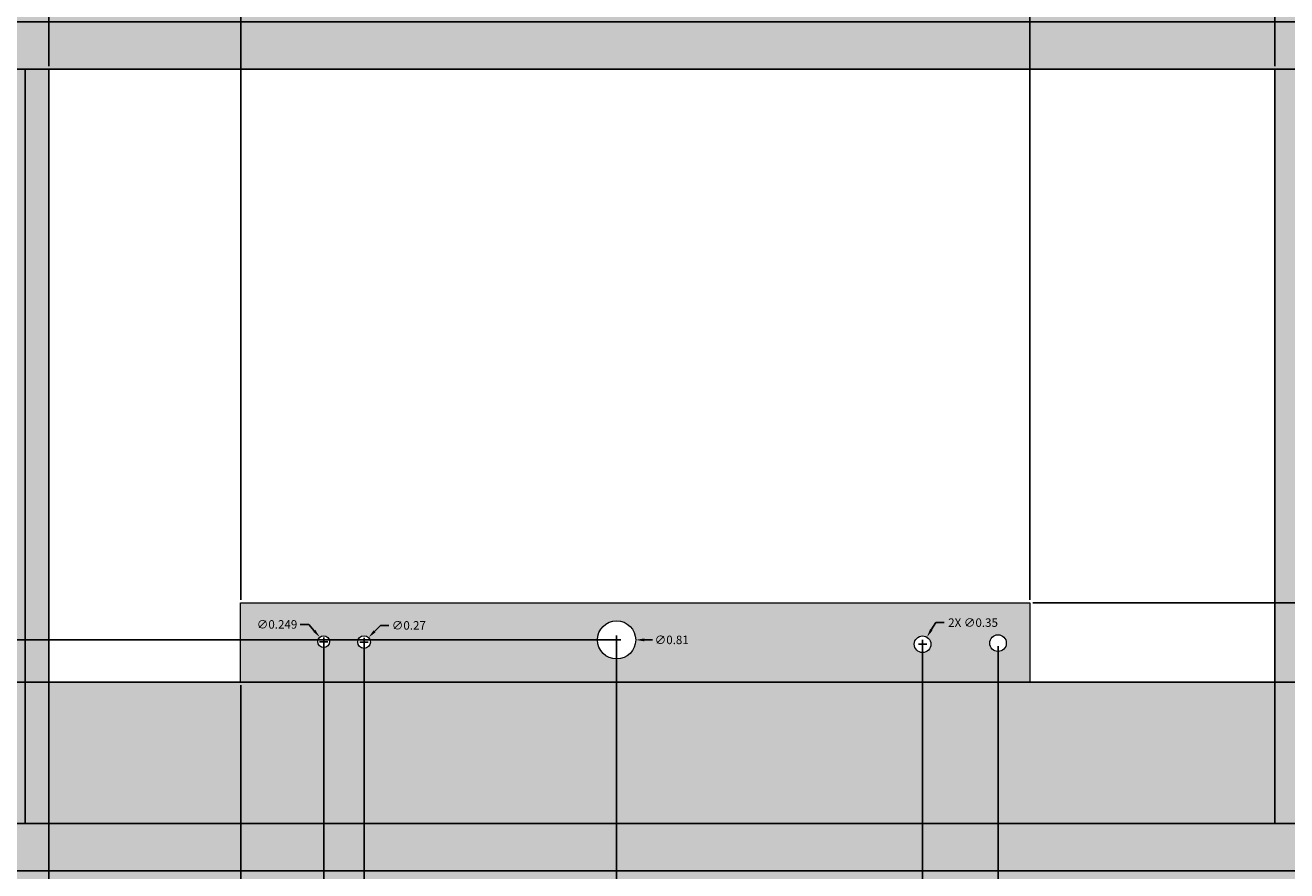
# Model space of a CAD drawing. Units: inches. Extents: x 4508 to 4723, y 847 to 1020.
# Tile 7 of 32: x 4604 to 4631, y 887 to 905. Entities that reach past the tile are written whole.
import ezdxf

# ---------------------------------------------------------------- set-up
doc = ezdxf.new("R2010")
doc.units = ezdxf.units.IN
for name, color, linetype, lineweight in [('A-ANNO-DIMS', 2, 'Continuous', 18), ('A-ANNO-NPLT', 8, 'Continuous', 13), ('A-EQPM', 4, 'Continuous', 18), ('A-FURN', 8, 'Continuous', 25), ('A-WALL-PATT', 254, 'Continuous', 13)]:
    doc.layers.add(name, color=color, linetype=linetype, lineweight=lineweight)
doc.styles.get("Standard").update_dxf_attribs({"font": 'arial.ttf'})
doc.dimstyles.get("Standard").update_dxf_attribs({"dimtxt": 0.18, "dimasz": 0.18, "dimexe": 0.18, "dimexo": 0.0625, "dimgap": 0.09, "dimtad": 0, "dimtih": 1, "dimtoh": 1, "dimdec": 4, "dimzin": 0, "dimdsep": 46, "dimtxsty": 'Standard', "dimcen": 0.09, "dimadec": 0, "dimazin": 0, "dimtfac": 1, "dimtdec": 4, "dimtofl": 0, "dimtmove": 0, "dimatfit": 3, "dimfxl": 1, "dimtolj": 1, "dimtzin": 0, "dimarcsym": 0})

# ---------------------------------------------------------------- blocks, each defined once
blk = doc.blocks.new('*D30')
at = {"layer": 'A-ANNO-DIMS', "color": 0, "lineweight": -2, "transparency": 16777216}
for p, q in [((4604.494, 903.809), (4604.494, 1002.877)), ((4630.494, 903.809), (4630.494, 1002.877)), ((4604.674, 1002.697), (4617.273, 1002.697)), ((4630.314, 1002.697), (4617.714, 1002.697))]:
    blk.add_line(p, q, dxfattribs=at)
at = {"layer": 'A-ANNO-DIMS', "color": 0, "lineweight": 9, "transparency": 16777216}
for points in [[(4604.674, 1002.727), (4604.674, 1002.667), (4604.494, 1002.697)], [(4630.314, 1002.727), (4630.314, 1002.667), (4630.494, 1002.697)]]:
    blk.add_solid(points, dxfattribs=at)
at = {"layer": 'Defpoints', "color": 0, "lineweight": 9, "transparency": 16777216}
for p in [(4630.494, 1002.697), (4604.494, 903.747), (4630.494, 903.747)]:
    blk.add_point(p, dxfattribs=at)
at = {"layer": 'A-ANNO-DIMS', "color": 0, "transparency": 16777216, "insert": (4617.494, 1002.697), "char_height": 0.18, "attachment_point": 5}
blk.add_mtext('\\A1;26', dxfattribs=at)
blk = doc.blocks.new('*D32')
at = {"layer": 'A-ANNO-DIMS', "color": 0, "lineweight": -2, "transparency": 16777216}
for p, q in [((4604.431, 890.747), (4532.864, 890.747)), ((4533.044, 890.567), (4533.044, 889.429)), ((4533.044, 887.927), (4533.044, 889.065)), ((4604.431, 887.747), (4532.864, 887.747))]:
    blk.add_line(p, q, dxfattribs=at)
at = {"layer": 'A-ANNO-DIMS', "color": 0, "lineweight": 9, "transparency": 16777216}
for points in [[(4533.014, 890.567), (4533.074, 890.567), (4533.044, 890.747)], [(4533.014, 887.927), (4533.074, 887.927), (4533.044, 887.747)]]:
    blk.add_solid(points, dxfattribs=at)
at = {"layer": 'Defpoints', "color": 0, "lineweight": 9, "transparency": 16777216}
for p in [(4533.044, 890.747), (4604.494, 890.747), (4604.494, 887.747)]:
    blk.add_point(p, dxfattribs=at)
at = {"layer": 'A-ANNO-DIMS', "color": 0, "transparency": 16777216, "insert": (4533.044, 889.247), "char_height": 0.18, "attachment_point": 5}
blk.add_mtext('\\A1;3', dxfattribs=at)
blk = doc.blocks.new('*D33')
at = {"layer": 'A-ANNO-DIMS', "color": 0, "lineweight": -2, "transparency": 16777216}
for p, q in [((4604.494, 890.684), (4604.494, 866.617)), ((4608.562, 890.684), (4608.562, 866.617)), ((4604.674, 866.797), (4606.13, 866.797)), ((4608.382, 866.797), (4606.925, 866.797))]:
    blk.add_line(p, q, dxfattribs=at)
at = {"layer": 'A-ANNO-DIMS', "color": 0, "lineweight": 9, "transparency": 16777216}
for points in [[(4604.674, 866.827), (4604.674, 866.767), (4604.494, 866.797)], [(4608.382, 866.827), (4608.382, 866.767), (4608.562, 866.797)]]:
    blk.add_solid(points, dxfattribs=at)
at = {"layer": 'Defpoints', "color": 0, "lineweight": 9, "transparency": 16777216}
for p in [(4604.494, 890.747), (4608.562, 890.747), (4608.562, 866.797)]:
    blk.add_point(p, dxfattribs=at)
at = {"layer": 'A-ANNO-DIMS', "color": 0, "transparency": 16777216, "insert": (4606.528, 866.797), "char_height": 0.18, "attachment_point": 5}
blk.add_mtext('\\A1;4.068', dxfattribs=at)
blk = doc.blocks.new('*D34')
at = {"layer": 'A-ANNO-DIMS', "color": 0, "lineweight": -2, "transparency": 16777216}
for p, q in [((4608.562, 892.49), (4608.562, 1002.877)), ((4625.298, 892.49), (4625.298, 1002.877)), ((4608.742, 1002.697), (4616.475, 1002.697)), ((4625.118, 1002.697), (4617.385, 1002.697))]:
    blk.add_line(p, q, dxfattribs=at)
at = {"layer": 'A-ANNO-DIMS', "color": 0, "lineweight": 9, "transparency": 16777216}
for points in [[(4608.742, 1002.727), (4608.742, 1002.667), (4608.562, 1002.697)], [(4625.118, 1002.727), (4625.118, 1002.667), (4625.298, 1002.697)]]:
    blk.add_solid(points, dxfattribs=at)
at = {"layer": 'Defpoints', "color": 0, "lineweight": 9, "transparency": 16777216}
for p in [(4625.298, 1002.697), (4608.562, 892.428), (4625.298, 892.428)]:
    blk.add_point(p, dxfattribs=at)
at = {"layer": 'A-ANNO-DIMS', "color": 0, "transparency": 16777216, "insert": (4616.93, 1002.697), "char_height": 0.18, "attachment_point": 5}
blk.add_mtext('\\A1;16.737', dxfattribs=at)
blk = doc.blocks.new('*D35')
at = {"layer": 'A-ANNO-DIMS', "color": 0, "lineweight": -2, "transparency": 16777216}
for p, q in [((4625.361, 892.428), (4702.124, 892.428)), ((4701.944, 892.248), (4701.944, 891.769)), ((4701.944, 890.927), (4701.944, 891.405)), ((4625.361, 890.747), (4702.124, 890.747))]:
    blk.add_line(p, q, dxfattribs=at)
at = {"layer": 'A-ANNO-DIMS', "color": 0, "lineweight": 9, "transparency": 16777216}
for points in [[(4701.914, 892.248), (4701.974, 892.248), (4701.944, 892.428)], [(4701.914, 890.927), (4701.974, 890.927), (4701.944, 890.747)]]:
    blk.add_solid(points, dxfattribs=at)
at = {"layer": 'Defpoints', "color": 0, "lineweight": 9, "transparency": 16777216}
for p in [(4625.298, 892.428), (4701.944, 892.428), (4625.298, 890.747)]:
    blk.add_point(p, dxfattribs=at)
at = {"layer": 'A-ANNO-DIMS', "color": 0, "transparency": 16777216, "insert": (4701.944, 891.587), "char_height": 0.18, "attachment_point": 5}
blk.add_mtext('\\A1;1.681', dxfattribs=at)
blk = doc.blocks.new('*D36')
at = {"layer": 'A-ANNO-DIMS', "color": 0, "lineweight": -2, "transparency": 16777216}
for p, q in [((4610.322, 891.543), (4610.322, 866.617)), ((4608.562, 890.684), (4608.562, 866.617)), ((4608.742, 866.797), (4609.127, 866.797)), ((4610.142, 866.797), (4609.757, 866.797))]:
    blk.add_line(p, q, dxfattribs=at)
at = {"layer": 'A-ANNO-DIMS', "color": 0, "lineweight": 9, "transparency": 16777216}
for points in [[(4608.742, 866.827), (4608.742, 866.767), (4608.562, 866.797)], [(4610.142, 866.827), (4610.142, 866.767), (4610.322, 866.797)]]:
    blk.add_solid(points, dxfattribs=at)
at = {"layer": 'Defpoints', "color": 0, "lineweight": 9, "transparency": 16777216}
for p in [(4610.322, 891.605), (4608.562, 890.747), (4610.322, 866.797)]:
    blk.add_point(p, dxfattribs=at)
at = {"layer": 'A-ANNO-DIMS', "color": 0, "transparency": 16777216, "insert": (4609.442, 866.797), "char_height": 0.18, "attachment_point": 5}
blk.add_mtext('\\A1;1.76', dxfattribs=at)
blk = doc.blocks.new('*D37')
at = {"layer": 'A-ANNO-DIMS', "color": 0, "lineweight": -2, "transparency": 16777216}
for p, q in [((4610.322248, 891.542903), (4610.322248, 866.616874)), ((4611.179162, 891.534506), (4611.179162, 866.616874)), ((4610.142248, 866.796874), (4609.962248, 866.796874)), ((4611.359162, 866.796874), (4611.539162, 866.796874))]:
    blk.add_line(p, q, dxfattribs=at)
at = {"layer": 'A-ANNO-DIMS', "color": 0, "lineweight": 9, "transparency": 16777216}
for points in [[(4610.142248, 866.826874), (4610.142248, 866.766874), (4610.322248, 866.796874)], [(4611.359162, 866.826874), (4611.359162, 866.766874), (4611.179162, 866.796874)]]:
    blk.add_solid(points, dxfattribs=at)
at = {"layer": 'Defpoints', "color": 0, "lineweight": 9, "transparency": 16777216}
for p in [(4610.322248, 891.605403), (4611.179162, 891.597006), (4611.179162, 866.796874)]:
    blk.add_point(p, dxfattribs=at)
at = {"layer": 'A-ANNO-DIMS', "color": 0, "transparency": 16777216, "insert": (4610.750705, 866.796874), "char_height": 0.18, "attachment_point": 5}
blk.add_mtext('\\A1;0.857', dxfattribs=at)
blk = doc.blocks.new('*D38')
at = {"layer": 'A-ANNO-DIMS', "color": 0, "lineweight": -2, "transparency": 16777216}
for p, q in [((4616.533, 891.581), (4616.533, 866.617)), ((4611.179, 891.535), (4611.179, 866.617)), ((4611.359, 866.797), (4613.463, 866.797)), ((4616.353, 866.797), (4614.249, 866.797))]:
    blk.add_line(p, q, dxfattribs=at)
at = {"layer": 'A-ANNO-DIMS', "color": 0, "lineweight": 9, "transparency": 16777216}
for points in [[(4611.359, 866.827), (4611.359, 866.767), (4611.179, 866.797)], [(4616.353, 866.827), (4616.353, 866.767), (4616.533, 866.797)]]:
    blk.add_solid(points, dxfattribs=at)
at = {"layer": 'Defpoints', "color": 0, "lineweight": 9, "transparency": 16777216}
for p in [(4611.179, 891.597), (4616.533, 891.643), (4616.533, 866.797)]:
    blk.add_point(p, dxfattribs=at)
at = {"layer": 'A-ANNO-DIMS', "color": 0, "transparency": 16777216, "insert": (4613.856, 866.797), "char_height": 0.18, "attachment_point": 5}
blk.add_mtext('\\A1;5.354', dxfattribs=at)
blk = doc.blocks.new('*D39')
at = {"layer": 'A-ANNO-DIMS', "color": 0, "lineweight": -2, "transparency": 16777216}
for p, q in [((4616.533, 891.581), (4616.533, 866.617)), ((4623.022, 891.488), (4623.022, 866.617)), ((4616.713, 866.797), (4619.383, 866.797)), ((4622.842, 866.797), (4620.172, 866.797))]:
    blk.add_line(p, q, dxfattribs=at)
at = {"layer": 'A-ANNO-DIMS', "color": 0, "lineweight": 9, "transparency": 16777216}
for points in [[(4616.713, 866.827), (4616.713, 866.767), (4616.533, 866.797)], [(4622.842, 866.827), (4622.842, 866.767), (4623.022, 866.797)]]:
    blk.add_solid(points, dxfattribs=at)
at = {"layer": 'Defpoints', "color": 0, "lineweight": 9, "transparency": 16777216}
for p in [(4616.533, 891.643), (4623.022, 891.551), (4623.022, 866.797)]:
    blk.add_point(p, dxfattribs=at)
at = {"layer": 'A-ANNO-DIMS', "color": 0, "transparency": 16777216, "insert": (4619.777, 866.797), "char_height": 0.18, "attachment_point": 5}
blk.add_mtext('\\A1;6.489', dxfattribs=at)
blk = doc.blocks.new('*D40')
at = {"layer": 'A-ANNO-DIMS', "color": 0, "lineweight": -2, "transparency": 16777216}
for p, q in [((4623.022, 891.488), (4623.022, 866.617)), ((4624.621, 891.511), (4624.621, 866.617)), ((4623.202, 866.797), (4623.436, 866.797)), ((4624.441, 866.797), (4624.207, 866.797))]:
    blk.add_line(p, q, dxfattribs=at)
at = {"layer": 'A-ANNO-DIMS', "color": 0, "lineweight": 9, "transparency": 16777216}
for points in [[(4623.202, 866.827), (4623.202, 866.767), (4623.022, 866.797)], [(4624.441, 866.827), (4624.441, 866.767), (4624.621, 866.797)]]:
    blk.add_solid(points, dxfattribs=at)
at = {"layer": 'Defpoints', "color": 0, "lineweight": 9, "transparency": 16777216}
for p in [(4623.022, 891.551), (4624.621, 891.574), (4624.621, 866.797)]:
    blk.add_point(p, dxfattribs=at)
at = {"layer": 'A-ANNO-DIMS', "color": 0, "transparency": 16777216, "insert": (4623.821, 866.797), "char_height": 0.18, "attachment_point": 5}
blk.add_mtext('\\A1;1.599', dxfattribs=at)
blk = doc.blocks.new('*D41')
at = {"layer": 'A-ANNO-DIMS', "color": 0, "lineweight": -2, "transparency": 16777216}
for p, q in [((4616.47, 891.643), (4532.864, 891.643)), ((4533.044, 891.643), (4533.044, 891.823)), ((4533.044, 891.823), (4533.224, 891.823)), ((4533.044, 890.927), (4533.044, 891.463)), ((4608.499, 890.747), (4532.864, 890.747))]:
    blk.add_line(p, q, dxfattribs=at)
at = {"layer": 'A-ANNO-DIMS', "color": 0, "lineweight": 9, "transparency": 16777216}
for points in [[(4533.014, 891.463), (4533.074, 891.463), (4533.044, 891.643)], [(4533.014, 890.927), (4533.074, 890.927), (4533.044, 890.747)]]:
    blk.add_solid(points, dxfattribs=at)
at = {"layer": 'Defpoints', "color": 0, "lineweight": 9, "transparency": 16777216}
for p in [(4533.044, 891.643), (4616.533, 891.643), (4608.562, 890.747)]:
    blk.add_point(p, dxfattribs=at)
at = {"layer": 'A-ANNO-DIMS', "color": 0, "transparency": 16777216, "insert": (4533.547, 891.823), "char_height": 0.18, "attachment_point": 5}
blk.add_mtext('\\A1;0.90', dxfattribs=at)
blk = doc.blocks.new('*D48')
at = {"layer": 'A-ANNO-DIMS', "color": 0, "lineweight": -2, "transparency": 16777216}
for p, q in [((4616.443, 891.643), (4616.623, 891.643)), ((4616.533, 891.553), (4616.533, 891.733)), ((4617.298, 891.643), (4617.118, 891.643))]:
    blk.add_line(p, q, dxfattribs=at)
at = {"layer": 'A-ANNO-DIMS', "color": 0, "lineweight": 9, "transparency": 16777216}
blk.add_solid([(4617.118, 891.673), (4617.118, 891.613), (4616.938, 891.643)], dxfattribs=at)
at = {"layer": 'Defpoints', "color": 0, "lineweight": 9, "transparency": 16777216}
for p in [(4616.128, 891.644), (4616.938, 891.643)]:
    blk.add_point(p, dxfattribs=at)
at = {"layer": 'A-ANNO-DIMS', "color": 0, "transparency": 16777216, "insert": (4617.702, 891.643), "char_height": 0.18, "attachment_point": 5}
blk.add_mtext('\\A1;∅0.81', dxfattribs=at)
blk = doc.blocks.new('*D49')
at = {"layer": 'A-ANNO-DIMS', "color": 0, "lineweight": -2, "transparency": 16777216}
for p, q in [((4609.824, 891.971), (4610.004, 891.971)), ((4610.004, 891.971), (4610.122, 891.835)), ((4610.232, 891.605), (4610.412, 891.605)), ((4610.322, 891.515), (4610.322, 891.695))]:
    blk.add_line(p, q, dxfattribs=at)
at = {"layer": 'A-ANNO-DIMS', "color": 0, "lineweight": 9, "transparency": 16777216}
blk.add_solid([(4610.145, 891.855), (4610.1, 891.816), (4610.241, 891.699)], dxfattribs=at)
at = {"layer": 'Defpoints', "color": 0, "lineweight": 9, "transparency": 16777216}
for p in [(4610.241, 891.699), (4610.404, 891.511)]:
    blk.add_point(p, dxfattribs=at)
at = {"layer": 'A-ANNO-DIMS', "color": 0, "transparency": 16777216, "insert": (4609.333, 891.971), "char_height": 0.18, "attachment_point": 5}
blk.add_mtext('\\A1;∅0.249', dxfattribs=at)
blk = doc.blocks.new('*D50')
at = {"layer": 'A-ANNO-DIMS', "color": 0, "lineweight": -2, "transparency": 16777216}
for p, q in [((4611.526, 891.95), (4611.4, 891.822)), ((4611.706, 891.95), (4611.526, 891.95)), ((4611.089, 891.597), (4611.269, 891.597)), ((4611.179, 891.507), (4611.179, 891.687))]:
    blk.add_line(p, q, dxfattribs=at)
at = {"layer": 'A-ANNO-DIMS', "color": 0, "lineweight": 9, "transparency": 16777216}
blk.add_solid([(4611.378, 891.843), (4611.421, 891.801), (4611.274, 891.693)], dxfattribs=at)
at = {"layer": 'Defpoints', "color": 0, "lineweight": 9, "transparency": 16777216}
for p in [(4611.274, 891.693), (4611.085, 891.501)]:
    blk.add_point(p, dxfattribs=at)
at = {"layer": 'A-ANNO-DIMS', "color": 0, "transparency": 16777216, "insert": (4612.128, 891.95), "char_height": 0.18, "attachment_point": 5}
blk.add_mtext('\\A1;∅0.27', dxfattribs=at)
blk = doc.blocks.new('*D51')
at = {"layer": 'A-ANNO-DIMS', "color": 0, "lineweight": -2, "transparency": 16777216}
for p, q in [((4623.299, 892.009), (4623.206, 891.855)), ((4623.479, 892.009), (4623.299, 892.009)), ((4623.022, 891.461), (4623.022, 891.641)), ((4622.932, 891.551), (4623.112, 891.551))]:
    blk.add_line(p, q, dxfattribs=at)
at = {"layer": 'A-ANNO-DIMS', "color": 0, "lineweight": 9, "transparency": 16777216}
blk.add_solid([(4623.181, 891.871), (4623.232, 891.84), (4623.113, 891.701)], dxfattribs=at)
at = {"layer": 'Defpoints', "color": 0, "lineweight": 9, "transparency": 16777216}
for p in [(4623.113, 891.701), (4622.93, 891.4)]:
    blk.add_point(p, dxfattribs=at)
at = {"layer": 'A-ANNO-DIMS', "color": 0, "transparency": 16777216, "insert": (4624.092, 892.009), "char_height": 0.18, "attachment_point": 5}
blk.add_mtext('\\A1;2X ∅0.35', dxfattribs=at)

msp = doc.modelspace()

# ---------------------------------------------------------------- hatches: boundary and pattern name
at = {"layer": 'A-WALL-PATT', "transparency": 33554508}
h = msp.add_hatch(color=256, dxfattribs=at)
h.dxf.hatch_style = 1
h.paths.add_polyline_path([(4661.6706, 954.043, -0.3739004), (4658.5765, 957.6021, -1), (4665.7646, 957.6021, -0.3739004), (4662.6706, 954.043), (4662.6706, 944.4021, -0.2114781), (4670.3062, 945.0869), (4670.3062, 968.0592, -0.4632086), (4663.3246, 973.9783, -0.4632086), (4670.3062, 979.8975), (4670.3062, 994.7469), (4588.9938, 994.7469), (4588.9938, 904.7469), (4657.9938, 904.7469), (4657.9938, 886.7469), (4549.9938, 886.7469), (4549.9938, 878.7469), (4693.9938, 878.7469), (4693.9938, 994.7469), (4671.8062, 994.7469), (4671.8062, 979.4411, -0.2941682), (4675.3246, 973.9783, -0.2941682), (4671.8062, 968.5156), (4671.8062, 944.4278, -0.2741114), (4676.7298, 936.1217, -0.2741114), (4671.8062, 927.8155), (4671.8062, 907.6998, -0.3779645), (4677.0562, 901.7469, -0.3779645), (4671.8062, 895.7939), (4671.8062, 883.7469), (4670.3062, 883.7469), (4670.3062, 895.7939, -0.3779645), (4665.0562, 901.7469, -0.3779645), (4670.3062, 907.6998), (4670.3062, 927.1564, -0.2114781), (4662.6706, 927.8412), (4662.6706, 918.2003, -0.3739004), (4665.7646, 914.6412, -1), (4658.5765, 914.6412, -0.3739004), (4661.6706, 918.2003), (4661.6706, 928.4807, -0.2391825), (4657.7936, 936.1217, -0.2391825), (4661.6706, 943.7626)])
at = {"layer": 'A-WALL-PATT', "transparency": 33554681}
h = msp.add_hatch(color=256, dxfattribs=at)
h.dxf.hatch_style = 1
h.paths.add_polyline_path([(4577.4938, 903.7469), (4550.9938, 903.7469), (4550.9938, 887.7469), (4577.4938, 887.7469)], flags=0)
h.paths.add_polyline_path([(4603.9938, 903.7469), (4577.9938, 903.7469), (4577.9938, 887.7469), (4603.9938, 887.7469)], flags=0)
h.paths.add_polyline_path([(4656.9938, 903.7469), (4630.9938, 903.7469), (4630.9938, 887.7469), (4656.9938, 887.7469)], flags=0)
h.paths.add_polyline_path([(4657.9938, 904.7469), (4549.9938, 904.7469), (4549.9938, 886.7469), (4657.9938, 886.7469)])
h.paths.add_polyline_path([(4656.9938, 903.7469), (4656.9938, 887.7469), (4550.9938, 887.7469), (4550.9938, 903.7469)], flags=16)
h = msp.add_hatch(color=256, dxfattribs=at)
h.dxf.hatch_style = 1
h.paths.add_polyline_path([(4577.4938, 903.7469), (4550.9938, 903.7469), (4550.9938, 887.7469), (4577.4938, 887.7469)])
h.paths.add_polyline_path([(4603.9938, 903.7469), (4577.9938, 903.7469), (4577.9938, 887.7469), (4603.9938, 887.7469)])
h.paths.add_polyline_path([(4656.9938, 903.7469), (4630.9938, 903.7469), (4630.9938, 887.7469), (4656.9938, 887.7469)])
h = msp.add_hatch(color=256, dxfattribs=at)
h.dxf.hatch_style = 1
h.paths.add_polyline_path([(4604.4938, 903.7469), (4603.9938, 903.7469), (4603.9938, 887.7469), (4604.4938, 887.7469)])
h.paths.add_polyline_path([(4630.9938, 903.7469), (4630.4938, 903.7469), (4630.4938, 887.7469), (4630.9938, 887.7469)])
h.paths.add_polyline_path([(4577.9938, 903.7469), (4577.4938, 903.7469), (4577.4938, 887.7469), (4577.9938, 887.7469)])
at = {"layer": 'A-WALL-PATT', "transparency": 33554676}
h = msp.add_hatch(color=256, dxfattribs=at)
h.dxf.hatch_style = 1
h.paths.add_polyline_path([(4625.2983, 892.4277), (4608.5617, 892.4277), (4608.5617, 890.7469), (4625.2983, 890.7469)])
h.paths.add_polyline_path([(4616.1277, 891.6433, -1), (4616.9379, 891.6433, -1)], flags=16)
h.paths.add_polyline_path([(4611.044, 891.597, -1), (4611.3143, 891.597, -1)], flags=16)
h.paths.add_polyline_path([(4610.1977, 891.6054, -1), (4610.4468, 891.6054, -1)], flags=16)
h.paths.add_polyline_path([(4623.198, 891.5507, -1), (4622.8455, 891.5507, -1)], flags=16)
h.paths.add_polyline_path([(4624.7971, 891.5739, -1), (4624.4444, 891.5739, -1)], flags=16)
at = {"layer": 'A-WALL-PATT', "transparency": 33554681}
h = msp.add_hatch(color=256, dxfattribs=at)
h.dxf.hatch_style = 1
h.paths.add_polyline_path([(4630.4938, 890.7469), (4604.4938, 890.7469), (4604.4938, 887.7469), (4630.4938, 887.7469)])

# ---------------------------------------------------------------- linework, layer by layer
at = {"layer": 'A-ANNO-NPLT'}
for p in [(4603.9938, 895.7469), (4630.4938, 895.7469)]:
    msp.add_point(p, dxfattribs=at)
at = {"layer": 'A-EQPM'}
msp.add_lwpolyline([(4608.5617, 892.4277), (4625.2983, 892.4277), (4625.2983, 890.7469), (4608.5617, 890.7469)], close=True, dxfattribs=at)
for centre, radius in [((4616.5328, 891.6433), 0.4051), ((4610.3222, 891.6054), 0.1245), ((4611.1792, 891.597), 0.1351), ((4623.0217, 891.5507), 0.1763), ((4624.6207, 891.5739), 0.1764)]:
    msp.add_circle(centre, radius, dxfattribs=at)
at = {"layer": 'A-FURN'}
for p, q in [((4603.9938, 903.7469), (4603.9938, 887.7469)), ((4604.4938, 903.7469), (4604.4938, 887.7469)), ((4630.4938, 903.7469), (4630.4938, 887.7469)), ((4604.4938, 890.7469), (4630.4938, 890.7469))]:
    msp.add_line(p, q, dxfattribs=at)
for points in [[(4657.9938, 886.7469), (4549.9938, 886.7469), (4549.9938, 904.7469), (4657.9938, 904.7469)], [(4656.9938, 887.7469), (4550.9938, 887.7469), (4550.9938, 903.7469), (4656.9938, 903.7469)]]:
    msp.add_lwpolyline(points, close=True, dxfattribs=at)

# ---------------------------------------------------------------- dimensions: what is measured, and where the dimension line sits
at = {"layer": 'A-ANNO-DIMS'}
for base, p1, p2, override, picture, middle in [((4630.4938, 1002.6969), (4604.4938, 903.7469), (4630.4938, 903.7469), {"dimdec": 0, "dimlfac": 1, "dimrnd": 0, "dimzin": 0, "dimdsep": 46, "dimlunit": 2}, '*D30', (4617.4938, 1002.6969)), ((4625.2983, 1002.6969), (4608.5617, 892.4277), (4625.2983, 892.4277), {"dimdec": 3, "dimlfac": 1, "dimrnd": 0, "dimzin": 0, "dimdsep": 46, "dimlunit": 2}, '*D34', (4616.93, 1002.6969)), ((4610.3222, 866.7969), (4608.5617, 890.7469), (4610.3222, 891.6054), {"dimdec": 2, "dimlfac": 1, "dimrnd": 0, "dimzin": 0, "dimdsep": 46, "dimlunit": 2}, '*D36', (4609.442, 866.7969)), ((4611.1792, 866.7969), (4610.3222, 891.6054), (4611.1792, 891.597), {"dimdec": 3, "dimlfac": 1, "dimrnd": 0, "dimzin": 0, "dimdsep": 46, "dimlunit": 2}, '*D37', (4610.7507, 866.7969)), ((4616.5328, 866.7969), (4611.1792, 891.597), (4616.5328, 891.6433), {"dimdec": 3, "dimlfac": 1, "dimrnd": 0, "dimzin": 0, "dimdsep": 46, "dimlunit": 2}, '*D38', (4613.856, 866.7969)), ((4623.0217, 866.7969), (4616.5328, 891.6433), (4623.0217, 891.5507), {"dimdec": 3, "dimlfac": 1, "dimrnd": 0, "dimzin": 0, "dimdsep": 46, "dimlunit": 2}, '*D39', (4619.7773, 866.7969)), ((4624.6207, 866.7969), (4623.0217, 891.5507), (4624.6207, 891.5739), {"dimdec": 3, "dimlfac": 1, "dimrnd": 0, "dimzin": 0, "dimdsep": 46, "dimlunit": 2}, '*D40', (4623.8212, 866.7969)), ((4608.5617, 866.7969), (4604.4938, 890.7469), (4608.5617, 890.7469), {"dimdec": 3, "dimlfac": 1, "dimrnd": 0, "dimzin": 0, "dimdsep": 46, "dimlunit": 2}, '*D33', (4606.5277, 866.7969))]:
    dim = msp.add_linear_dim(base=base, p1=p1, p2=p2, dimstyle='Standard', override=override, dxfattribs=at)
    dim.commit()
    dim.dimension.update_dxf_attribs({"geometry": picture, "text_midpoint": middle})
for base, p1, p2, override, picture, middle in [((4701.9438, 892.4277), (4625.2983, 890.7469), (4625.2983, 892.4277), {"dimdec": 3, "dimlfac": 1, "dimrnd": 0, "dimzin": 0, "dimdsep": 46, "dimlunit": 2}, '*D35', (4701.9438, 891.5873)), ((4533.0438, 891.6433), (4608.5617, 890.7469), (4616.5328, 891.6433), {"dimdec": 2, "dimlfac": 1, "dimrnd": 0, "dimzin": 0, "dimdsep": 46, "dimlunit": 2}, '*D41', (4533.5473, 891.8233)), ((4533.0438, 890.7469), (4604.4938, 887.7469), (4604.4938, 890.7469), {"dimdec": 0, "dimlfac": 1, "dimrnd": 0, "dimzin": 0, "dimdsep": 46, "dimlunit": 2}, '*D32', (4533.0438, 889.2469))]:
    dim = msp.add_linear_dim(base=base, p1=p1, p2=p2, angle=90, dimstyle='Standard', override=override, dxfattribs=at)
    dim.commit()
    dim.dimension.update_dxf_attribs({"geometry": picture, "text_midpoint": middle})
dim = msp.add_diameter_dim_2p(p1=(4622.9305, 891.3999), p2=(4623.113, 891.7015), text='2X <>', dimstyle='Standard', override={"dimdec": 2, "dimlfac": 1, "dimrnd": 0, "dimzin": 0, "dimdsep": 46, "dimlunit": 2}, dxfattribs=at)
dim.commit()
dim.dimension.update_dxf_attribs({"geometry": '*D51', "text_midpoint": (4624.0919, 892.0095), "dimtype": 163})
for p1, p2, override, picture, middle in [((4610.4039, 891.5114), (4610.2406, 891.6994), {"dimdec": 3, "dimlfac": 1, "dimrnd": 0, "dimzin": 0, "dimdsep": 46, "dimlunit": 2}, '*D49', (4609.3325, 891.971)), ((4611.0845, 891.5005), (4611.2738, 891.6935), {"dimdec": 2, "dimlfac": 1, "dimrnd": 0, "dimzin": 0, "dimdsep": 46, "dimlunit": 2}, '*D50', (4612.1276, 891.9505))]:
    dim = msp.add_diameter_dim_2p(p1=p1, p2=p2, dimstyle='Standard', override=override, dxfattribs=at)
    dim.commit()
    dim.dimension.update_dxf_attribs({"geometry": picture, "text_midpoint": middle, "dimtype": 163})
dim = msp.add_diameter_dim_2p(p1=(4616.1277, 891.6437), p2=(4616.9379, 891.643), dimstyle='Standard', override={"dimdec": 2, "dimlfac": 1, "dimrnd": 0, "dimzin": 0, "dimdsep": 46, "dimlunit": 2}, dxfattribs=at)
dim.commit()
dim.dimension.update_dxf_attribs({"geometry": '*D48', "text_midpoint": (4617.2979, 891.6427)})

doc.saveas('drawing.dxf')
